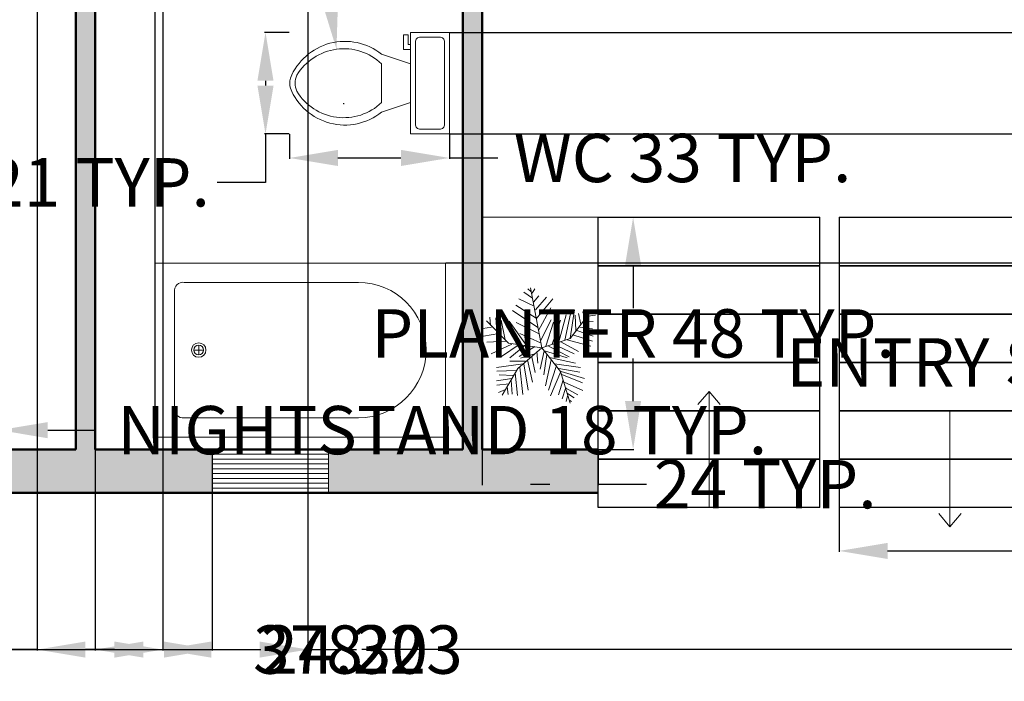
# Model space of a CAD drawing. Units: inches. Extents: x 133 to 758, y -29 to 543.
# Tile 2 of 7: x 386 to 590, y -29 to 108. Entities that reach past the tile are written whole.
import ezdxf

# ---------------------------------------------------------------- set-up
doc = ezdxf.new("R2010")
doc.units = ezdxf.units.IN
doc.header["$MEASUREMENT"] = 0
for name, color, linetype, lineweight in [('A-ANNO-DIMS', 2, 'Continuous', 18), ('A-ANNO-SYMB', 7, 'Continuous', 18), ('A-FLOR-FIXT', 9, 'Continuous', 20), ('A-FLOR-STRS', 7, 'Continuous', 25), ('A-WALL', 7, 'Continuous', 50), ('PLANT', 72, 'Continuous', 18), ('WINDOW', 151, 'Continuous', 18)]:
    doc.layers.add(name, color=color, linetype=linetype, lineweight=lineweight)
doc.layers.add('A-WALL-PATT', color=251, linetype='Continuous', lineweight=13, true_color=0x636466)
doc.styles.get("Standard").update_dxf_attribs({"font": 'arial.ttf'})
doc.dimstyles.get("Standard").update_dxf_attribs({"dimtxt": 10, "dimasz": 10, "dimexe": 0.18, "dimexo": 0.0625, "dimgap": 0.09, "dimtad": 0, "dimtih": 1, "dimtoh": 1, "dimdec": 0, "dimzin": 0, "dimdsep": 46, "dimlunit": 4, "dimtxsty": 'Standard', "dimcen": 0.09, "dimadec": 0, "dimazin": 0, "dimtfac": 1, "dimtdec": 0, "dimtofl": 0, "dimtmove": 0, "dimatfit": 3, "dimfxl": 1, "dimtolj": 1, "dimtzin": 0, "dimarcsym": 0})

# ---------------------------------------------------------------- blocks, each defined once
blk = doc.blocks.new('*U16')
for p, q in [((0, 0), (-266.7, 1447.8)), ((-221.9198, 1197.3052), (-433.5526, 1338.8594)), ((-258.7244, 1362.456), (-332.3336, 1421.4348)), ((-231.1146, 1315.2628), (-166.7002, 1421.4348)), ((-194.31, 1102.9442), (-65.4812, 1256.284)), ((-148.3106, 914.1968), (118.5418, 1220.9018)), ((-129.8956, 713.6638), (-626.7704, 1032.1544)), ((-185.1152, 1008.5578), (-553.1612, 1185.4942)), ((-129.8956, 701.8528), (265.7602, 1185.4942)), ((-74.7014, 418.7444), (219.7608, 961.39)), ((-1234.059, 536.7274), (-1252.4486, 737.2604)), ((-1105.2302, 725.4494), (-1077.6458, 395.1732)), ((-902.8176, 713.6638), (-617.5756, 100.2538)), ((-93.091, 489.5342), (-700.3796, 902.3858)), ((412.9786, 147.447), (587.8068, 796.2392)), ((560.197, 182.8292), (698.2206, 819.8358)), ((685.8, 228.6), (1219.2, 914.4)), ((689.0258, 230.0224), (790.2448, 914.1968)), ((808.6344, 784.4282), (827.0494, 418.7444)), ((891.4384, 831.6214), (946.658, 572.1096)), ((983.4626, 867.0036), (1066.2666, 725.4494)), ((1112.2914, 760.8316), (1296.3144, 784.4282)), ((1121.4862, 925.9824), (1149.0706, 831.6214)), ((-1206.4492, 501.3198), (-1418.082, 465.9376)), ((-800.1, 114.3), (-1333.5, 647.7)), ((-976.4268, 666.4706), (-884.4026, 194.6402)), ((-369.1382, 53.086), (-783.1836, 642.874)), ((-617.5756, 607.4918), (-74.7014, 347.98)), ((-28.6766, 171.0436), (228.9556, 678.2816)), ((100.1268, 41.275), (284.1498, 619.2774)), ((256.5654, 88.4682), (449.7832, 666.4706)), ((919.0482, 501.3198), (1222.6798, 454.152)), ((1029.462, 654.685), (1241.0948, 631.0884)), ((-1031.621, 347.98), (-1399.667, 277.1902)), ((-525.5514, 347.98), (-28.6766, 123.8504)), ((753.4148, 312.5978), (1222.6798, 159.2326)), ((845.439, 418.7444), (1241.0948, 277.1902)), ((-847.598, 159.2326), (-1326.0578, 135.636)), ((-718.7946, 88.4682), (-1215.644, -147.447)), ((-543.9664, 76.6572), (-967.2066, -206.4512)), ((0, 0), (-800.1, 114.3)), ((-405.9428, 53.086), (-764.794, -241.8334)), ((0, 0), (-571.5, -495.3)), ((-166.7002, 29.4894), (-543.9664, -206.4512)), ((0, 0), (685.8, 228.6)), ((0, 0), (457.2, -571.5)), ((164.5412, 41.275), (661.416, -218.2368)), ((284.1498, 88.4682), (781.0246, -147.447)), ((458.978, 147.447), (891.4384, -88.4682)), ((615.4166, 194.6402), (1185.8752, 41.275)), ((-166.7002, -147.447), (-507.1618, -253.619)), ((-240.3094, -218.2368), (-157.5054, -595.7062)), ((-120.7008, -88.4682), (-93.091, -371.5766)), ((63.3222, -76.6826), (-37.8714, -513.1308)), ((44.9326, -64.897), (615.4166, -241.8334)), ((127.7366, -159.258), (54.1274, -654.685)), ((192.151, -230.0224), (817.8292, -371.5766)), ((-442.7474, -383.3876), (-1086.8406, -477.7486)), ((-387.5278, -324.4088), (-764.794, -324.4088)), ((-525.5514, -465.963), (-451.9422, -1126.5408)), ((-433.5526, -383.3876), (-323.1134, -1020.3688)), ((-341.5284, -289.0012), (-221.9198, -831.6214)), ((228.9556, -289.0012), (90.932, -914.1968)), ((357.759, -430.5554), (164.5412, -1020.3688)), ((311.7596, -383.3876), (937.4378, -477.7486)), ((-617.5756, -548.5384), (-1077.6458, -560.324)), ((-681.9646, -666.496), (-1022.4262, -654.685)), ((-571.5, -495.3), (-952.5, -1143)), ((-635.9652, -607.5172), (-580.771, -1150.1374)), ((458.978, -572.1096), (210.5406, -1161.923)), ((412.9786, -501.3452), (919.0482, -583.9206)), ((457.2, -571.5), (685.8, -1333.5)), ((468.1982, -572.1096), (1029.462, -737.2604)), ((486.5878, -642.8994), (983.4626, -843.4324)), ((-718.7946, -737.2604), (-1086.8406, -796.2392)), ((-783.1836, -867.029), (-1077.6458, -902.4112)), ((-829.2084, -937.7934), (-810.7934, -1126.5408)), ((-737.1842, -784.4536), (-709.5744, -1114.7298)), ((514.1976, -772.6426), (403.7838, -1138.3264)), ((541.8074, -831.6214), (992.6574, -1032.1544)), ((-875.2078, -1008.5832), (-1040.8412, -1079.3476)), ((578.612, -961.39), (495.7826, -1232.7128)), ((578.612, -973.1756), (873.0488, -1138.3264)), ((624.6114, -1161.923), (587.8068, -1291.6916)), ((624.6114, -1102.9442), (781.0246, -1209.1162)), ((679.8056, -1268.095), (716.6102, -1291.6916))]:
    blk.add_line(p, q)
blk = doc.blocks.new('Bath Tub - 26 x 60 in.')
for p, q in [((8, -18), (10, -18)), ((9, -17), (9, -19))]:
    blk.add_line(p, q)
blk.add_lwpolyline([(0, -36), (0, 0), (60, 0), (60, -36)], close=True)
for points in [[(6, -4), (42, -4)], [(4, -30), (4, -6)], [(42, -32), (6, -32)]]:
    blk.add_lwpolyline(points)
for radius in [1.5, 1]:
    blk.add_circle((9, -18), radius)
for centre, radius, start, end in [((5.75, -5.75), 1.77, 81.8699, 188.1301), ((42, -18), 14, 270, 90), ((5.75, -30.25), 1.77, 171.8699, 278.1301)]:
    blk.add_arc(centre, radius, start, end)
blk = doc.blocks.new('Toilet - top')
for p, q in [((9.5, -6), (9.5, -2)), ((-8, -8.5), (-8, -8)), ((-7, -8), (-7, -9.5)), ((-4, -8), (-6, -14)), ((4, -8), (6, -14)), ((-10, -8.5), (-8, -8.5)), ((-10, -9.5), (-10, -8.5)), ((-7, -9.5), (-10, -9.5)), ((4, -14), (-4, -14))]:
    blk.add_line(p, q)
blk.add_lwpolyline([(10.5, -8), (10.5, 0), (-10.5, 0), (-10.5, -8)], close=True)
for points in [[(-9.5, -2), (-9.5, -6)], [(8.5, -1), (-8.5, -1)], [(-8.5, -7), (8.5, -7)]]:
    blk.add_lwpolyline(points)
for centre, radius, start, end in [((-8.62, -1.88), 0.884, 81.8699, 188.1301), ((8.62, -1.88), 0.884, 351.8699, 98.1301), ((-8.62, -6.12), 0.884, 171.8699, 278.1301), ((8.62, -6.12), 0.884, 261.8699, 8.1301), ((3.52, -21.58), 12.17, 141.4691, 247.9714), ((4.2, -21.82), 11.33, 136.3677, 238.9468), ((-3.52, -21.58), 12.17, 292.0284, 38.5307), ((-4.2, -21.82), 11.33, 301.053, 43.6321), ((0, -27.88), 4, 245.7318, 294.2682), ((0, -29), 4, 254.8605, 285.1395)]:
    blk.add_arc(centre, radius, start, end)
blk = doc.blocks.new('WIN-24IN')
for p, q in [((0, 8), (24, 8)), ((0, 7), (24, 7)), ((0, 6), (24, 6)), ((0, 5), (24, 5)), ((0, 4), (24, 4)), ((0, 3), (24, 3)), ((0, 2), (24, 2)), ((0, 1), (24, 1))]:
    blk.add_line(p, q)
blk.add_lwpolyline([(24, 9), (24, 0), (0, 0), (0, 9)], close=True)
blk = doc.blocks.new('PORCH-STAIR-6-TREAD')
blk.add_line((0, 60), (0, 0))
for points in [[(0, 60), (45.8, 60), (45.8, 50), (0, 50)], [(0, 50), (45.8, 50), (45.8, 40), (0, 40)], [(0, 40), (45.8, 40), (45.8, 30), (0, 30)], [(0, 30), (45.8, 30), (45.8, 20), (0, 20)], [(0, 20), (45.8, 20), (45.8, 10), (0, 10)], [(0, 10), (45.8, 10), (45.8, 0), (0, 0)]]:
    blk.add_lwpolyline(points)
blk = doc.blocks.new('STAIR-DIRECTION')
for p, q in [((2.33, 24), (0, 21.27)), ((2.33, 0), (2.33, 24)), ((2.33, 24), (4.65, 21.27))]:
    blk.add_line(p, q)
blk = doc.blocks.new('PLANTER-24X48IN')
blk.add_lwpolyline([(0, 0), (24, 0), (24, 48), (0, 48)], close=True)
blk = doc.blocks.new('*D40')
at = {"layer": 'A-ANNO-DIMS', "color": 0, "lineweight": -2, "transparency": 16777216}
for p, q in [((363.97, 25.96), (363.97, 23.14)), ((381.97, 25.96), (381.97, 23.14)), ((353.97, 23.32), (343.97, 23.32)), ((391.97, 23.32), (401.97, 23.32))]:
    blk.add_line(p, q, dxfattribs=at)
at = {"layer": 'A-ANNO-DIMS', "color": 0, "transparency": 16777216}
for points in [[(353.97, 24.99), (353.97, 21.65), (363.97, 23.32)], [(391.97, 24.99), (391.97, 21.65), (381.97, 23.32)]]:
    blk.add_solid(points, dxfattribs=at)
at = {"layer": 'Defpoints', "color": 0, "transparency": 16777216}
for p in [(363.97, 26.02), (381.97, 26.02), (381.97, 23.32)]:
    blk.add_point(p, dxfattribs=at)
at = {"layer": 'A-ANNO-DIMS', "color": 0, "transparency": 16777216, "insert": (473.5, 23.32), "char_height": 10, "attachment_point": 5}
blk.add_mtext('\\A1;NIGHTSTAND 18 TYP.', dxfattribs=at)
blk = doc.blocks.new('*D50')
at = {"layer": 'A-ANNO-DIMS', "color": 0, "lineweight": -2, "transparency": 16777216}
for p, q in [((441.92, 84.51), (441.92, 79.43)), ((474.97, 84.51), (474.97, 79.43)), ((451.92, 79.61), (464.97, 79.61)), ((474.97, 79.61), (484.97, 79.61))]:
    blk.add_line(p, q, dxfattribs=at)
at = {"layer": 'A-ANNO-DIMS', "color": 0, "transparency": 16777216}
for points in [[(451.92, 81.28), (451.92, 77.95), (441.92, 79.61)], [(464.97, 81.28), (464.97, 77.95), (474.97, 79.61)]]:
    blk.add_solid(points, dxfattribs=at)
at = {"layer": 'Defpoints', "color": 0, "transparency": 16777216}
for p in [(441.92, 84.57), (474.97, 84.57), (474.97, 79.61)]:
    blk.add_point(p, dxfattribs=at)
at = {"layer": 'A-ANNO-DIMS', "color": 0, "transparency": 16777216, "insert": (523.18, 79.61), "char_height": 10, "attachment_point": 5}
blk.add_mtext('\\A1;WC 33 TYP.', dxfattribs=at)
blk = doc.blocks.new('*D51')
at = {"layer": 'A-ANNO-DIMS', "color": 0, "lineweight": -2, "transparency": 16777216}
for p, q in [((441.86, 105.57), (436.79, 105.57)), ((436.97, 95.57), (436.97, 94.57)), ((441.86, 84.57), (436.79, 84.57)), ((436.97, 84.57), (436.97, 74.57)), ((436.97, 74.57), (426.97, 74.57))]:
    blk.add_line(p, q, dxfattribs=at)
at = {"layer": 'A-ANNO-DIMS', "color": 0, "transparency": 16777216}
for points in [[(435.3, 95.57), (438.63, 95.57), (436.97, 105.57)], [(435.3, 94.57), (438.63, 94.57), (436.97, 84.57)]]:
    blk.add_solid(points, dxfattribs=at)
at = {"layer": 'Defpoints', "color": 0, "transparency": 16777216}
for p in [(441.92, 105.57), (436.97, 84.57), (441.92, 84.57)]:
    blk.add_point(p, dxfattribs=at)
at = {"layer": 'A-ANNO-DIMS', "color": 0, "transparency": 16777216, "insert": (402.45, 74.57), "char_height": 10, "attachment_point": 5}
blk.add_mtext('\\A1;21 TYP.', dxfattribs=at)
blk = doc.blocks.new('*D58')
at = {"layer": 'A-ANNO-DIMS', "color": 0, "lineweight": -2, "transparency": 16777216}
for p, q in [((601.41, 67.34), (610.53, 67.34)), ((610.35, 57.34), (610.35, 42.6)), ((610.35, 17.34), (610.35, 32.08)), ((601.41, 7.34), (610.53, 7.34))]:
    blk.add_line(p, q, dxfattribs=at)
at = {"layer": 'A-ANNO-DIMS', "color": 0, "transparency": 16777216}
for points in [[(608.68, 57.34), (612.02, 57.34), (610.35, 67.34)], [(608.68, 17.34), (612.02, 17.34), (610.35, 7.34)]]:
    blk.add_solid(points, dxfattribs=at)
at = {"layer": 'Defpoints', "color": 0, "transparency": 16777216}
for p in [(601.35, 67.34), (610.35, 67.34), (601.35, 7.34)]:
    blk.add_point(p, dxfattribs=at)
at = {"layer": 'A-ANNO-DIMS', "color": 0, "transparency": 16777216, "insert": (610.35, 37.34), "char_height": 10, "attachment_point": 5}
blk.add_mtext('\\A1;ENTRY STAIR 60 TYP.', dxfattribs=at)
blk = doc.blocks.new('*D59')
at = {"layer": 'A-ANNO-DIMS', "color": 0, "lineweight": -2, "transparency": 16777216}
for p, q in [((555.55, 7.27), (555.55, -1.84)), ((601.35, 7.27), (601.35, -1.84)), ((565.55, -1.66), (591.35, -1.66)), ((601.35, -1.66), (611.35, -1.66))]:
    blk.add_line(p, q, dxfattribs=at)
at = {"layer": 'A-ANNO-DIMS', "color": 0, "transparency": 16777216}
for points in [[(565.55, 0), (565.55, -3.33), (555.55, -1.66)], [(591.35, 0), (591.35, -3.33), (601.35, -1.66)]]:
    blk.add_solid(points, dxfattribs=at)
at = {"layer": 'Defpoints', "color": 0, "transparency": 16777216}
for p in [(555.55, 7.34), (601.35, 7.34), (601.35, -1.66)]:
    blk.add_point(p, dxfattribs=at)
at = {"layer": 'A-ANNO-DIMS', "color": 0, "transparency": 16777216, "insert": (635.98, -1.66), "char_height": 10, "attachment_point": 5}
blk.add_mtext('\\A1;46 TYP.', dxfattribs=at)
blk = doc.blocks.new('*D60')
at = {"layer": 'A-ANNO-DIMS', "color": 0, "lineweight": -2, "transparency": 16777216}
for p, q in [((505.81, 67.34), (513.13, 67.34)), ((512.95, 57.34), (512.95, 48.53)), ((512.95, 29.34), (512.95, 38.14)), ((505.81, 19.34), (513.13, 19.34))]:
    blk.add_line(p, q, dxfattribs=at)
at = {"layer": 'A-ANNO-DIMS', "color": 0, "transparency": 16777216}
for points in [[(511.28, 57.34), (514.62, 57.34), (512.95, 67.34)], [(511.28, 29.34), (514.62, 29.34), (512.95, 19.34)]]:
    blk.add_solid(points, dxfattribs=at)
at = {"layer": 'Defpoints', "color": 0, "transparency": 16777216}
for p in [(505.75, 67.34), (512.95, 67.34), (505.75, 19.34)]:
    blk.add_point(p, dxfattribs=at)
at = {"layer": 'A-ANNO-DIMS', "color": 0, "transparency": 16777216, "insert": (512.95, 43.34), "char_height": 10, "attachment_point": 5}
blk.add_mtext('\\A1;PLANTER 48 TYP.', dxfattribs=at)
blk = doc.blocks.new('*D61')
at = {"layer": 'A-ANNO-DIMS', "color": 0, "lineweight": -2, "transparency": 16777216}
for p, q in [((481.75, 19.27), (481.75, 11.96)), ((505.75, 19.27), (505.75, 11.96)), ((491.75, 12.14), (495.75, 12.14)), ((505.75, 12.14), (515.75, 12.14))]:
    blk.add_line(p, q, dxfattribs=at)
at = {"layer": 'A-ANNO-DIMS', "color": 0, "transparency": 16777216}
for points in [[(491.75, 13.8), (491.75, 10.47), (481.75, 12.14)], [(495.75, 13.8), (495.75, 10.47), (505.75, 12.14)]]:
    blk.add_solid(points, dxfattribs=at)
at = {"layer": 'Defpoints', "color": 0, "transparency": 16777216}
for p in [(481.75, 19.34), (505.75, 19.34), (505.75, 12.14)]:
    blk.add_point(p, dxfattribs=at)
at = {"layer": 'A-ANNO-DIMS', "color": 0, "transparency": 16777216, "insert": (540.26, 12.14), "char_height": 10, "attachment_point": 5}
blk.add_mtext('\\A1;24 TYP.', dxfattribs=at)
blk = doc.blocks.new('*D72')
at = {"layer": 'A-ANNO-DIMS', "color": 0, "lineweight": -2, "transparency": 16777216}
for p, q in [((256.75, 10.27), (256.75, -22.24)), ((634.75, 10.27), (634.75, -22.24)), ((266.75, -22.06), (434.61, -22.06)), ((624.75, -22.06), (456.89, -22.06))]:
    blk.add_line(p, q, dxfattribs=at)
at = {"layer": 'A-ANNO-DIMS', "color": 0, "transparency": 16777216}
for points in [[(266.75, -20.4), (266.75, -23.73), (256.75, -22.06)], [(624.75, -20.4), (624.75, -23.73), (634.75, -22.06)]]:
    blk.add_solid(points, dxfattribs=at)
at = {"layer": 'Defpoints', "color": 0, "transparency": 16777216}
for p in [(256.75, 10.34), (634.75, 10.34), (634.75, -22.06)]:
    blk.add_point(p, dxfattribs=at)
at = {"layer": 'A-ANNO-DIMS', "color": 0, "transparency": 16777216, "insert": (445.75, -22.06), "char_height": 10, "attachment_point": 5}
blk.add_mtext('\\A1;378', dxfattribs=at)
blk = doc.blocks.new('*D84')
at = {"layer": 'A-ANNO-DIMS', "color": 0, "lineweight": -2, "transparency": 16777216}
for p, q in [((401.75, 19.27), (401.75, -22.24)), ((425.97, 19.27), (425.97, -22.24)), ((411.75, -22.06), (415.97, -22.06)), ((425.97, -22.06), (435.97, -22.06))]:
    blk.add_line(p, q, dxfattribs=at)
at = {"layer": 'A-ANNO-DIMS', "color": 0, "transparency": 16777216}
for points in [[(411.75, -20.4), (411.75, -23.73), (401.75, -22.06)], [(415.97, -20.4), (415.97, -23.73), (425.97, -22.06)]]:
    blk.add_solid(points, dxfattribs=at)
at = {"layer": 'Defpoints', "color": 0, "transparency": 16777216}
for p in [(401.75, 19.34), (425.97, 19.34), (425.97, -22.06)]:
    blk.add_point(p, dxfattribs=at)
at = {"layer": 'A-ANNO-DIMS', "color": 0, "transparency": 16777216, "insert": (456.91, -22.06), "char_height": 10, "attachment_point": 5}
blk.add_mtext('\\A1;24.223', dxfattribs=at)
blk = doc.blocks.new('*D85')
at = {"layer": 'A-ANNO-DIMS', "color": 0, "lineweight": -2, "transparency": 16777216}
for p, q in [((389.75, 399.27), (389.75, -22.24)), ((415.75, 399.27), (415.75, -22.24)), ((389.75, -22.06), (379.75, -22.06)), ((405.75, -22.06), (399.75, -22.06))]:
    blk.add_line(p, q, dxfattribs=at)
at = {"layer": 'A-ANNO-DIMS', "color": 0, "transparency": 16777216}
for points in [[(399.75, -20.4), (399.75, -23.73), (389.75, -22.06)], [(405.75, -20.4), (405.75, -23.73), (415.75, -22.06)]]:
    blk.add_solid(points, dxfattribs=at)
at = {"layer": 'Defpoints', "color": 0, "transparency": 16777216}
for p in [(389.75, 399.34), (415.75, 399.34), (389.75, -22.06)]:
    blk.add_point(p, dxfattribs=at)
at = {"layer": 'A-ANNO-DIMS', "color": 0, "transparency": 16777216, "insert": (372.42, -22.06), "char_height": 10, "attachment_point": 5}
blk.add_mtext('\\A1;26', dxfattribs=at)
blk = doc.blocks.new('*D91')
at = {"layer": 'A-ANNO-DIMS', "color": 0, "lineweight": -2, "transparency": 16777216}
for p, q in [((415.75, 399.27), (415.75, -22.24)), ((445.75, 399.27), (445.75, -22.24)), ((425.75, -22.06), (435.75, -22.06)), ((445.75, -22.06), (455.75, -22.06))]:
    blk.add_line(p, q, dxfattribs=at)
at = {"layer": 'A-ANNO-DIMS', "color": 0, "transparency": 16777216}
for points in [[(425.75, -20.4), (425.75, -23.73), (415.75, -22.06)], [(435.75, -20.4), (435.75, -23.73), (445.75, -22.06)]]:
    blk.add_solid(points, dxfattribs=at)
at = {"layer": 'Defpoints', "color": 0, "transparency": 16777216}
for p in [(415.75, 399.34), (445.75, 399.34), (445.75, -22.06)]:
    blk.add_point(p, dxfattribs=at)
at = {"layer": 'A-ANNO-DIMS', "color": 0, "transparency": 16777216, "insert": (462.98, -22.06), "char_height": 10, "attachment_point": 5}
blk.add_mtext('\\A1;30', dxfattribs=at)
blk = doc.blocks.new('*D93')
at = {"layer": 'A-ANNO-DIMS', "color": 0, "lineweight": -2, "transparency": 16777216}
for p, q in [((477.81, 163.34), (660.33, 163.34)), ((660.15, 153.34), (660.15, 139.65)), ((660.15, 115.57), (660.15, 129.26)), ((475.03, 105.57), (660.33, 105.57))]:
    blk.add_line(p, q, dxfattribs=at)
at = {"layer": 'A-ANNO-DIMS', "color": 0, "transparency": 16777216}
for points in [[(658.48, 153.34), (661.82, 153.34), (660.15, 163.34)], [(658.48, 115.57), (661.82, 115.57), (660.15, 105.57)]]:
    blk.add_solid(points, dxfattribs=at)
at = {"layer": 'Defpoints', "color": 0, "transparency": 16777216}
for p in [(477.75, 163.34), (660.15, 163.34), (474.97, 105.57)]:
    blk.add_point(p, dxfattribs=at)
at = {"layer": 'A-ANNO-DIMS', "color": 0, "transparency": 16777216, "insert": (660.15, 134.45), "char_height": 10, "attachment_point": 5}
blk.add_mtext('\\A1;57.76', dxfattribs=at)
blk = doc.blocks.new('*D94')
at = {"layer": 'A-ANNO-DIMS', "color": 0, "lineweight": -2, "transparency": 16777216}
for p, q in [((660.15, 84.57), (660.15, 94.57)), ((660.15, 94.57), (670.15, 94.57)), ((475.03, 84.57), (660.33, 84.57)), ((660.15, 67.89), (660.15, 74.57)), ((474.23, 57.89), (660.33, 57.89))]:
    blk.add_line(p, q, dxfattribs=at)
at = {"layer": 'A-ANNO-DIMS', "color": 0, "transparency": 16777216}
for points in [[(658.48, 74.57), (661.82, 74.57), (660.15, 84.57)], [(658.48, 67.89), (661.82, 67.89), (660.15, 57.89)]]:
    blk.add_solid(points, dxfattribs=at)
at = {"layer": 'Defpoints', "color": 0, "transparency": 16777216}
for p in [(474.97, 84.57), (660.15, 84.57), (474.17, 57.89)]:
    blk.add_point(p, dxfattribs=at)
at = {"layer": 'A-ANNO-DIMS', "color": 0, "transparency": 16777216, "insert": (691.12, 94.57), "char_height": 10, "attachment_point": 5}
blk.add_mtext('\\A1;26.685', dxfattribs=at)
blk = doc.blocks.new('*D99')
at = {"layer": 'A-ANNO-DIMS', "color": 0, "lineweight": -2, "transparency": 16777216}
for p, q in [((391.75, 533.74), (381.75, 533.74)), ((401.75, 19.4), (401.75, 533.92)), ((414.17, 21.95), (414.17, 533.92)), ((424.17, 533.74), (434.17, 533.74))]:
    blk.add_line(p, q, dxfattribs=at)
at = {"layer": 'A-ANNO-DIMS', "color": 0, "transparency": 16777216}
for points in [[(391.75, 535.4), (391.75, 532.07), (401.75, 533.74)], [(424.17, 535.4), (424.17, 532.07), (414.17, 533.74)]]:
    blk.add_solid(points, dxfattribs=at)
at = {"layer": 'Defpoints', "color": 0, "transparency": 16777216}
for p in [(401.75, 533.74), (414.17, 21.89), (401.75, 19.34)]:
    blk.add_point(p, dxfattribs=at)
at = {"layer": 'A-ANNO-DIMS', "color": 0, "transparency": 16777216, "insert": (361.37, 533.74), "char_height": 10, "attachment_point": 5}
blk.add_mtext('\\A1;12.417', dxfattribs=at)
blk = doc.blocks.new('*D102')
at = {"layer": 'A-ANNO-DIMS', "color": 0, "lineweight": -2, "transparency": 16777216}
for p, q in [((438.98, 121.92), (448.98, 121.92)), ((448.98, 121.92), (450.31, 112.01)), ((453.06, 90.87), (453.24, 90.87)), ((453.15, 90.78), (453.15, 90.96))]:
    blk.add_line(p, q, dxfattribs=at)
at = {"layer": 'A-ANNO-DIMS', "color": 0, "transparency": 16777216}
blk.add_solid([(451.96, 112.23), (448.66, 111.79), (451.64, 102.1)], dxfattribs=at)
at = {"layer": 'Defpoints', "color": 0, "transparency": 16777216}
for p in [(451.64, 102.1), (453.15, 90.87)]:
    blk.add_point(p, dxfattribs=at)
at = {"layer": 'A-ANNO-DIMS', "color": 0, "transparency": 16777216, "insert": (406.29, 121.92), "char_height": 10, "attachment_point": 5}
blk.add_mtext('\\A1;4X R11.33', dxfattribs=at)

msp = doc.modelspace()

# ---------------------------------------------------------------- hatches: boundary and pattern name
at = {"layer": 'A-WALL-PATT'}
h = msp.add_hatch(color=256, dxfattribs=at)
h.dxf.hatch_style = 1
h.paths.add_polyline_path([(425.9734, 19.336), (401.7501, 19.336), (401.7501, 163.336), (403.7501, 163.336), (403.7501, 167.336), (391.7501, 167.336), (391.7501, 163.336), (397.7501, 163.336), (397.7501, 19.336), (357.4362, 19.336), (357.4362, 10.336), (425.9734, 10.336)])
h = msp.add_hatch(color=256, dxfattribs=at)
h.dxf.hatch_style = 1
h.paths.add_polyline_path([(505.7501, 17.336), (505.7501, 19.336), (481.7501, 19.336), (481.7501, 67.336), (481.7501, 163.336), (481.7501, 167.336), (433.7501, 167.336), (433.7501, 163.336), (477.7501, 163.336), (477.7501, 19.336), (449.9734, 19.336), (449.9734, 10.336), (505.7501, 10.336)])

# ---------------------------------------------------------------- linework, layer by layer
at = {"layer": 'A-WALL'}
for p, q in [((397.7501, 19.336), (397.7501, 163.336)), ((401.7501, 19.336), (401.7501, 163.336)), ((477.7501, 19.336), (477.7501, 163.336)), ((481.7501, 19.336), (481.7501, 163.336)), ((397.7501, 19.336), (265.7501, 19.336)), ((477.7501, 19.336), (401.7501, 19.336)), ((505.7501, 19.336), (481.7501, 19.336))]:
    msp.add_line(p, q, dxfattribs=at)
msp.add_lwpolyline([(505.7501, 10.336), (256.7501, 10.336), (256.7501, 508.336), (634.7501, 508.336), (634.7501, 10.336), (601.3503, 10.336)], dxfattribs=at)

# ---------------------------------------------------------------- block references
at = {"layer": 'A-ANNO-SYMB'}
msp.add_blockref('STAIR-DIRECTION', (526.325, 7.336), dxfattribs=at)
at = {"layer": 'A-ANNO-SYMB', "rotation": 180}
msp.add_blockref('STAIR-DIRECTION', (580.7754, 27.3361), dxfattribs=at)
at = {"layer": 'A-FLOR-FIXT', "rotation": 270}
msp.add_blockref('Toilet - top', (474.9703, 95.0711), dxfattribs=at)
at = {"layer": 'A-FLOR-FIXT'}
msp.add_blockref('Bath Tub - 26 x 60 in.', (414.1676, 57.886), dxfattribs=at)
at = {"layer": 'A-FLOR-STRS', "rotation": 180}
msp.add_blockref('PORCH-STAIR-6-TREAD', (551.5504, 67.3361), dxfattribs=at)
at = {"layer": 'A-FLOR-STRS'}
msp.add_blockref('PORCH-STAIR-6-TREAD', (555.55, 7.336), dxfattribs=at)
at = {"layer": 'PLANT'}
msp.add_blockref('PLANTER-24X48IN', (481.75, 19.336), dxfattribs=at)
at = {"layer": 'PLANT', "xscale": 0.0085716703265903, "yscale": 0.0085716703265903, "zscale": 0.0085716703265903}
msp.add_blockref('*U16', (494.0549, 40.3482), dxfattribs=at)
at = {"layer": 'WINDOW'}
msp.add_blockref('WIN-24IN', (425.9733, 10.336), dxfattribs=at)

# ---------------------------------------------------------------- dimensions: what is measured, and where the dimension line sits
at = {"layer": 'A-ANNO-DIMS'}
for base, p1, p2, override, picture, middle in [((401.75012, 533.73604), (414.16755, 21.88596), (401.75012, 19.33604), {"dimdec": 3, "dimlfac": 1, "dimrnd": 0, "dimzin": 0, "dimdsep": 46, "dimlunit": 2}, '*D99', (361.37362, 533.73604)), ((389.7501, -22.064), (415.7501, 399.336), (389.7501, 399.336), {"dimdec": 0, "dimlfac": 1, "dimrnd": 0, "dimzin": 0, "dimdsep": 46, "dimlunit": 2}, '*D85', (372.4159, -22.064)), ((445.7501, -22.064), (415.7501, 399.336), (445.7501, 399.336), {"dimdec": 0, "dimlfac": 1, "dimrnd": 0, "dimzin": 0, "dimdsep": 46, "dimlunit": 2}, '*D91', (462.982, -22.064)), ((425.9734, -22.064), (401.7501, 19.336), (425.9734, 19.336), {"dimdec": 3, "dimlfac": 1, "dimrnd": 0, "dimzin": 0, "dimdsep": 46, "dimlunit": 2}, '*D84', (456.9058, -22.064)), ((634.7501, -22.064), (256.7501, 10.336), (634.7501, 10.336), {"dimdec": 0, "dimlfac": 1, "dimrnd": 0, "dimzin": 0, "dimdsep": 46, "dimlunit": 2}, '*D72', (445.7501, -22.064))]:
    dim = msp.add_linear_dim(base=base, p1=p1, p2=p2, dimstyle='Standard', override=override, dxfattribs=at)
    dim.commit()
    dim.dimension.update_dxf_attribs({"geometry": picture, "text_midpoint": middle})
for base, p1, p2, override, picture, middle in [((660.1501, 163.336), (474.9703, 105.5711), (477.7501, 163.336), {"dimdec": 2, "dimlfac": 1, "dimrnd": 0, "dimzin": 0, "dimdsep": 46, "dimlunit": 2}, '*D93', (660.1501, 134.4536)), ((660.1501, 84.5711), (474.1676, 57.886), (474.9703, 84.5711), {"dimdec": 3, "dimlfac": 1, "dimrnd": 0, "dimzin": 0, "dimdsep": 46, "dimlunit": 2}, '*D94', (691.1201, 94.5711))]:
    dim = msp.add_linear_dim(base=base, p1=p1, p2=p2, angle=90, dimstyle='Standard', override=override, dxfattribs=at)
    dim.commit()
    dim.dimension.update_dxf_attribs({"geometry": picture, "text_midpoint": middle})
dim = msp.add_radius_dim(center=(453.1529, 90.8712), mpoint=(451.643, 102.0993), text='4X <>', dimstyle='Standard', override={"dimdec": 2, "dimlfac": 1, "dimrnd": 0, "dimzin": 0, "dimdsep": 46, "dimlunit": 2}, dxfattribs=at)
dim.commit()
dim.dimension.update_dxf_attribs({"geometry": '*D102', "text_midpoint": (406.2851, 121.9209)})
for base, p1, p2, angle, text, picture, middle in [((436.9671, 84.5711), (441.924, 105.5711), (441.924, 84.5711), 270, '<> TYP.', '*D51', (402.4535, 74.5711)), ((512.9501, 67.336), (505.7501, 19.336), (505.7501, 67.336), 90, 'PLANTER <> TYP.', '*D60', (512.9501, 43.336)), ((610.3503, 67.336), (601.3503, 7.336), (601.3503, 67.336), 90, 'ENTRY STAIR <> TYP.', '*D58', (610.3503, 37.336)), ((381.9667, 23.3197), (363.9667, 26.0197), (381.9667, 26.0197), 0, 'NIGHTSTAND <> TYP.', '*D40', (473.496, 23.3197))]:
    dim = msp.add_linear_dim(base=base, p1=p1, p2=p2, angle=angle, text=text, dimstyle='Standard', override={"dimdec": 0, "dimlfac": 1, "dimrnd": 0, "dimzin": 0, "dimdsep": 46, "dimlunit": 2}, dxfattribs=at)
    dim.commit()
    dim.dimension.update_dxf_attribs({"geometry": picture, "text_midpoint": middle})
for base, p1, p2, text, picture, middle in [((474.9703, 79.6142), (441.924, 84.5711), (474.9703, 84.5711), 'WC <> TYP.', '*D50', (523.181, 79.6142)), ((505.7501, 12.136), (481.7501, 19.336), (505.7501, 19.336), '<> TYP.', '*D61', (540.2637, 12.136)), ((601.3503, -1.664), (555.5502, 7.336), (601.3503, 7.336), '<> TYP.', '*D59', (635.9799, -1.664))]:
    dim = msp.add_linear_dim(base=base, p1=p1, p2=p2, text=text, dimstyle='Standard', override={"dimdec": 0, "dimlfac": 1, "dimrnd": 0, "dimzin": 0, "dimdsep": 46, "dimlunit": 2}, dxfattribs=at)
    dim.commit()
    dim.dimension.update_dxf_attribs({"geometry": picture, "text_midpoint": middle})

doc.saveas('drawing.dxf')
